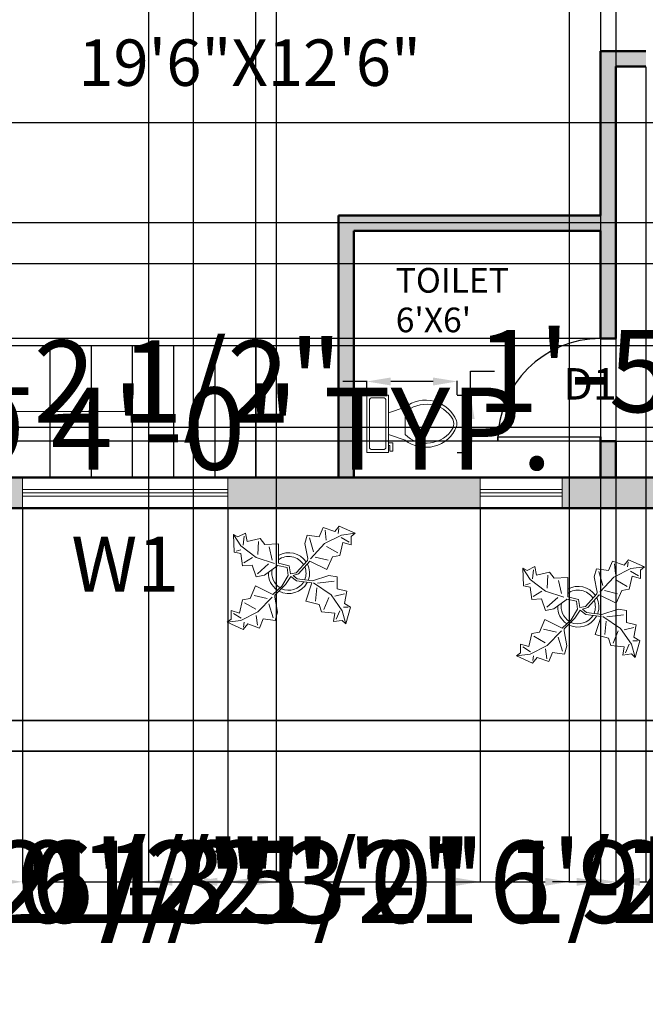
# Model space of a CAD drawing. Units: inches. Extents: x -166 to 1001, y 0 to 688.
# Tile 3 of 11: x 224 to 406, y 0 to 287. Entities that reach past the tile are written whole.
import ezdxf

# ---------------------------------------------------------------- set-up
doc = ezdxf.new("R2010")
doc.units = ezdxf.units.IN
doc.header["$MEASUREMENT"] = 0
for name, color, linetype, lineweight in [('A-ANNO-DIMS', 1, 'Continuous', 18), ('A-ANNO-SYMB', 7, 'Continuous', 18), ('A-ANNO-TEXT', 2, 'Continuous', 25), ('A-AREA-IDEN', 2, 'Continuous', 25), ('A-DOOR', 6, 'Continuous', 25), ('A-FLOR-FIXT', 11, 'Continuous', 18), ('A-FLOR-STRS', 7, 'Continuous', 25), ('A-GLAZ', 130, 'Continuous', 18), ('A-GLAZ-VENT', 130, 'Continuous', 18), ('A-WALL-PATT', 5, 'Continuous', 13), ('C-SITE-WALL', 250, 'Continuous', 35), ('TREES', 80, 'Continuous', 13), ('WALLS', 250, 'Continuous', 50)]:
    doc.layers.add(name, color=color, linetype=linetype, lineweight=lineweight)
doc.styles.get("Standard").update_dxf_attribs({"font": 'arial.ttf'})
doc.dimstyles.get("Standard").update_dxf_attribs({"dimtxt": 24, "dimasz": 7, "dimexe": 0.18, "dimexo": 0.0625, "dimgap": 0.09, "dimtad": 0, "dimtih": 1, "dimtoh": 1, "dimdec": 0, "dimzin": 0, "dimdsep": 46, "dimlunit": 3, "dimtxsty": 'Standard', "dimcen": 0.09, "dimadec": 0, "dimazin": 0, "dimtfac": 1, "dimtdec": 0, "dimtofl": 0, "dimtmove": 0, "dimatfit": 3, "dimfxl": 1, "dimtolj": 1, "dimtzin": 0, "dimarcsym": 0})

# ---------------------------------------------------------------- blocks, each defined once
blk = doc.blocks.new('*U6')
for p, q in [((0, 0), (0, -6)), ((40, 0), (40, -6))]:
    blk.add_line(p, q)
blk.add_lwpolyline([(0, 0), (0, 40), (1.75, 40), (1.75, 0)], close=True)
blk.add_arc((0, 0), 40, 0, 90)
blk = doc.blocks.new('Toilet - top')
for p, q in [((9.5, -6), (9.5, -2)), ((-10, -8.5), (-8, -8.5)), ((-10, -9.5), (-10, -8.5)), ((-7, -9.5), (-10, -9.5)), ((-8, -8.5), (-8, -8)), ((-7, -8), (-7, -9.5)), ((-4, -8), (-6, -14)), ((4, -8), (6, -14)), ((4, -14), (-4, -14))]:
    blk.add_line(p, q)
blk.add_lwpolyline([(10.5, -8), (10.5, 0), (-10.5, 0), (-10.5, -8)], close=True)
for points in [[(-9.5, -2), (-9.5, -6)], [(8.5, -1), (-8.5, -1)], [(-8.5, -7), (8.5, -7)]]:
    blk.add_lwpolyline(points)
for centre, radius, start, end in [((-8.62, -1.88), 0.884, 81.8699, 188.1301), ((8.62, -1.88), 0.884, 351.8699, 98.1301), ((-8.62, -6.12), 0.884, 171.8699, 278.1301), ((8.62, -6.12), 0.884, 261.8699, 8.1301), ((3.52, -21.58), 12.17, 141.4691, 247.9714), ((4.2, -21.82), 11.33, 136.3677, 238.9468), ((-3.52, -21.58), 12.17, 292.0284, 38.5307), ((-4.2, -21.82), 11.33, 301.053, 43.6321), ((0, -27.88), 4, 245.7318, 294.2682), ((0, -29), 4, 254.8605, 285.1395)]:
    blk.add_arc(centre, radius, start, end)
blk = doc.blocks.new('Plant - Rubber or Philodendron')
for p, q in [((-14.8639, 10.7964), (-12.6195, 11.8975)), ((-12.6195, 11.8975), (-12.1909, 9.4345)), ((8.8871, 10.7908), (9.9809, 13.4933)), ((9.9809, 13.4933), (13.3837, 12.301)), ((10.5828, 12.6946), (10.8893, 9.7953)), ((13.3837, 12.301), (14.68, 13.9039)), ((14.5816, 13.2037), (14.3848, 11.8033)), ((14.68, 13.9039), (19.3848, 11.8146)), ((19.3848, 11.8146), (15.3859, 11.3055)), ((19.3848, 11.8146), (18.1868, 10.9119)), ((-16.2005, 11.4774), (-13.9899, 8.1064)), ((-16.2005, 11.4774), (-14.8639, 10.7964)), ((-16.0159, 6.3329), (-16.2005, 11.4774)), ((-13.3174, 8.325), (-13.0735, 11.0065)), ((-12.1909, 9.4345), (-8.3829, 10.3)), ((-8.8369, 9.409), (-9.0894, 5.6095)), ((-8.3829, 10.3), (-7.0549, 8.501)), ((-7.0549, 8.501), (-3.0284, 8.6941)), ((-3.0284, 8.6941), (-3.0709, 3.1041)), ((4.6914, 8.8812), (5.3859, 11.2828)), ((4.6914, 8.8812), (5.5014, 4.4831)), ((5.3859, 11.2828), (8.8871, 10.7908)), ((5.9878, 10.4842), (7.1971, 6.3869)), ((10.3916, 8.7942), (6.2847, 4.4028)), ((15.3859, 11.3055), (10.3916, 8.7942)), ((15.7909, 9.1065), (14.8995, 5.3044)), ((15.2875, 10.6053), (17.5907, 9.2105)), ((18.1925, 8.4119), (15.7909, 9.1065)), ((18.1868, 10.9119), (18.1925, 8.4119)), ((-14.0069, 5.8704), (-16.0159, 6.3329)), ((-15.3434, 6.5514), (-13.9984, 6.9884)), ((-13.5868, 2.2894), (-14.0069, 5.8704)), ((-13.9899, 8.1064), (-9.5434, 4.7185)), ((-4.8529, 4.012), (-5.7184, 7.82)), ((14.2977, 6.1031), (10.9934, 7.9956)), ((-13.1329, 3.1804), (-10.6614, 4.727)), ((-9.5434, 4.7185), (-4.1917, 2.9888)), ((-9.1318, 0.0195), (-5.9793, 2.9025)), ((-3.0709, 3.1041), (0.0797, 2.3163)), ((2.1141, 0.2298), (5.4346, 3.9146)), ((6.1032, 3.6844), (2.8262, -0.031)), ((5.4346, 3.9146), (5.5014, 4.4831)), ((11.1089, 1.1958), (6.1032, 3.6844)), ((7.7005, 4.8881), (11.5025, 3.9967)), ((12.7005, 4.8994), (11.1089, 1.1958)), ((14.8995, 5.3044), (12.7005, 4.8994)), ((-10.6784, 2.491), (-13.5868, 2.2894)), ((-9.5858, -0.8715), (-10.6784, 2.491)), ((-7.1228, -0.443), (-3.5248, 2.2131)), ((-3.5248, 2.2131), (-3.3011, 2.4355)), ((-3.3011, 2.4355), (-0.5306, 1.7947)), ((-0.5306, 1.7947), (-0.2255, -0.5527)), ((-0.5306, 1.7947), (-0.5306, 1.7947)), ((0.0797, 2.3163), (0.4866, -0.031)), ((0.4866, -0.031), (2.1141, 0.2298)), ((-7.1228, -0.443), (-9.5858, -0.8715)), ((-2.019, -3.6148), (-0.2255, -0.5527)), ((-0.9375, -3.1608), (0.5883, -0.8135)), ((0.5883, -0.8135), (2.2447, -2.0916)), ((2.8262, -0.031), (1.3003, -0.5527)), ((1.3003, -0.5527), (2.4193, -1.4655)), ((2.2447, -2.0916), (6.7108, -2.6626)), ((2.4193, -1.4655), (6.895, -2.1175)), ((4.943, -7.9659), (6.7108, -2.6626)), ((11.6605, -0.5413), (6.895, -2.1175)), ((12.3677, -6.1981), (7.219, -2.6772)), ((8.3544, -2.7453), (13.1973, -2.1704)), ((11.6605, -0.5413), (14.1354, -0.8948)), ((14.1354, -0.8948), (14.1354, -4.4304)), ((-11.3237, -7.2629), (-9.7321, -3.5593)), ((-9.7321, -3.5593), (-4.7264, -6.0479)), ((-2.019, -3.6148), (-4.7264, -6.0479)), ((-4.0579, -6.2781), (-0.9375, -3.1608)), ((8.125, -4.0768), (7.7715, -7.9659)), ((14.1354, -4.4304), (16.9638, -5.1375)), ((16.9638, -5.1375), (16.2567, -8.673)), ((-14.4141, -11.4699), (-13.5228, -7.6679)), ((-13.5228, -7.6679), (-11.3237, -7.2629)), ((-12.921, -8.4665), (-9.6166, -10.359)), ((-6.3237, -7.2516), (-10.1257, -6.3602)), ((-9.0148, -11.1577), (-4.9047, -6.8122)), ((-4.1246, -6.8466), (-4.0579, -6.2781)), ((-3.3146, -11.2447), (-4.1246, -6.8466)), ((8.8321, -9.0266), (4.943, -7.9659)), ((10.2463, -10.4408), (11.6605, -6.9053)), ((15.5496, -10.7943), (12.3677, -6.1981)), ((16.2567, -5.8446), (13.4283, -6.5517)), ((-16.8157, -10.7754), (-14.4141, -11.4699)), ((-16.8101, -13.2754), (-16.8157, -10.7754)), ((-14.0091, -13.669), (-9.0148, -11.1577)), ((-4.611, -12.8477), (-5.8203, -8.7504)), ((-3.3146, -11.2447), (-4.0092, -13.6463)), ((9.5392, -11.1479), (8.8321, -9.0266)), ((13.4283, -11.5015), (9.5392, -11.1479)), ((13.0748, -13.9763), (13.4283, -11.5015)), ((14.8425, -10.7943), (13.7819, -13.2692)), ((16.6103, -14.6834), (15.5496, -10.7943)), ((17.3174, -9.7337), (15.9032, -9.7337)), ((16.2567, -8.673), (18.0245, -9.7337)), ((18.0245, -9.7337), (16.6103, -14.6834)), ((-18.008, -14.1781), (-16.8101, -13.2754)), ((-18.008, -14.1781), (-14.0091, -13.669)), ((-13.3032, -16.2674), (-18.008, -14.1781)), ((-13.9107, -12.9688), (-16.2139, -11.574)), ((-13.2048, -15.5672), (-13.008, -14.1668)), ((-9.206, -15.0581), (-9.5126, -12.1588)), ((-7.5103, -13.1543), (-8.6042, -15.8568)), ((-4.0092, -13.6463), (-7.5103, -13.1543)), ((15.5496, -13.6228), (13.0748, -13.9763)), ((16.6103, -14.6834), (15.5496, -13.6228)), ((-12.0069, -14.6645), (-13.3032, -16.2674)), ((-8.6042, -15.8568), (-12.0069, -14.6645))]:
    blk.add_line(p, q)
for centre, radius, start, end in [((0, 0), 6.1275, 34.37569, 120.1028), ((-0.0601, -0.2075), 5.2461, 33.82192, 124.9414), ((0.0308, 0.1664), 6, 178.6147, 235.1169), ((0.0308, 0.1664), 5, 168.1647, 238.6725), ((-0.2664, 0.1682), 5.2775, 338.4094, 20.03007), ((-0.098, 0.1364), 6.1288, 341.2017, 26.09184), ((-0.0234, 0.3825), 6.1492, 242.5812, 331.2714), ((-0.1102, 0.4886), 5.2883, 247.3711, 327.472)]:
    blk.add_arc(centre, radius, start, end)
blk = doc.blocks.new('VENT-24IN')
for p, q in [((0, 4.5), (0, 9)), ((0, 9), (0, 0)), ((24, 9), (24, 0)), ((0, 5.5), (24, 5.5)), ((0, 4.5), (24, 4.5)), ((0, 3.5), (24, 3.5))]:
    blk.add_line(p, q)
blk = doc.blocks.new('*D23')
at = {"layer": 'A-ANNO-DIMS', "color": 0, "lineweight": -2, "transparency": 16777216}
for p, q in [((103.92, 175.12), (103.92, 167.8)), ((151.92, 175.12), (151.92, 167.8)), ((110.92, 167.98), (144.92, 167.98)), ((151.92, 167.98), (158.92, 167.98))]:
    blk.add_line(p, q, dxfattribs=at)
at = {"layer": 'A-ANNO-DIMS', "color": 0, "transparency": 16777216}
for points in [[(110.92, 169.15), (110.92, 166.82), (103.92, 167.98)], [(144.92, 169.15), (144.92, 166.82), (151.92, 167.98)]]:
    blk.add_solid(points, dxfattribs=at)
at = {"layer": 'Defpoints', "color": 0, "transparency": 16777216}
for p in [(103.92, 175.18), (151.92, 175.18), (151.92, 167.98)]:
    blk.add_point(p, dxfattribs=at)
at = {"layer": 'A-ANNO-DIMS', "color": 0, "transparency": 16777216, "insert": (270.75, 167.98), "char_height": 24, "attachment_point": 5}
blk.add_mtext('\\A1;BED 4\'-0" TYP.', dxfattribs=at)
blk = doc.blocks.new('*D27')
at = {"layer": 'A-ANNO-DIMS', "color": 0, "lineweight": -2, "transparency": 16777216}
for p, q in [((325.13, 181.76), (318.13, 181.76)), ((325.13, 177.86), (325.13, 181.94)), ((344.51, 181.76), (332.13, 181.76)), ((351.51, 177.86), (351.51, 181.94))]:
    blk.add_line(p, q, dxfattribs=at)
at = {"layer": 'A-ANNO-DIMS', "color": 0, "transparency": 16777216}
for points in [[(332.13, 182.92), (332.13, 180.59), (325.13, 181.76)], [(344.51, 182.92), (344.51, 180.59), (351.51, 181.76)]]:
    blk.add_solid(points, dxfattribs=at)
at = {"layer": 'Defpoints', "color": 0, "transparency": 16777216}
for p in [(325.13, 181.76), (325.13, 177.8), (351.51, 177.8)]:
    blk.add_point(p, dxfattribs=at)
at = {"layer": 'A-ANNO-DIMS', "color": 0, "transparency": 16777216, "insert": (225.11, 181.76), "char_height": 24, "attachment_point": 5}
blk.add_mtext('\\A1;WC 2\'-2 1/2"', dxfattribs=at)
blk = doc.blocks.new('*D28')
at = {"layer": 'A-ANNO-DIMS', "color": 0, "lineweight": -2, "transparency": 16777216}
for p, q in [((355.46, 177.8), (355.46, 184.8)), ((355.46, 184.8), (362.46, 184.8)), ((351.57, 177.8), (355.64, 177.8)), ((355.46, 168.04), (355.46, 170.8)), ((351.57, 161.04), (355.64, 161.04))]:
    blk.add_line(p, q, dxfattribs=at)
at = {"layer": 'A-ANNO-DIMS', "color": 0, "transparency": 16777216}
for points in [[(354.29, 170.8), (356.63, 170.8), (355.46, 177.8)], [(354.29, 168.04), (356.63, 168.04), (355.46, 161.04)]]:
    blk.add_solid(points, dxfattribs=at)
at = {"layer": 'Defpoints', "color": 0, "transparency": 16777216}
for p in [(351.51, 177.8), (355.46, 177.8), (351.51, 161.04)]:
    blk.add_point(p, dxfattribs=at)
at = {"layer": 'A-ANNO-DIMS', "color": 0, "transparency": 16777216, "insert": (393.32, 184.8), "char_height": 24, "attachment_point": 5}
blk.add_mtext('\\A1;1\'-5"', dxfattribs=at)
blk = doc.blocks.new('*D42')
at = {"layer": 'A-ANNO-DIMS', "color": 0, "lineweight": -2, "transparency": 16777216}
for p, q in [((224.58, 144.68), (224.58, 35.41)), ((284.58, 144.68), (284.58, 35.41)), ((231.58, 35.59), (277.58, 35.59)), ((284.58, 35.59), (291.58, 35.59))]:
    blk.add_line(p, q, dxfattribs=at)
at = {"layer": 'A-ANNO-DIMS', "color": 0, "transparency": 16777216}
for points in [[(231.58, 36.76), (231.58, 34.42), (224.58, 35.59)], [(277.58, 36.76), (277.58, 34.42), (284.58, 35.59)]]:
    blk.add_solid(points, dxfattribs=at)
at = {"layer": 'Defpoints', "color": 0, "transparency": 16777216}
for p in [(224.58, 144.74), (284.58, 144.74), (284.58, 35.59)]:
    blk.add_point(p, dxfattribs=at)
at = {"layer": 'A-ANNO-DIMS', "color": 0, "transparency": 16777216, "insert": (323.57, 35.59), "char_height": 24, "attachment_point": 5}
blk.add_mtext('\\A1;5\'-0"', dxfattribs=at)
blk = doc.blocks.new('*D43')
at = {"layer": 'A-ANNO-DIMS', "color": 0, "lineweight": -2, "transparency": 16777216}
for p, q in [((160.88, 257.49), (160.88, 593.07)), ((167.88, 592.89), (201.62, 592.89)), ((208.62, 257.49), (208.62, 593.07)), ((208.62, 592.89), (215.62, 592.89))]:
    blk.add_line(p, q, dxfattribs=at)
at = {"layer": 'A-ANNO-DIMS', "color": 0, "transparency": 16777216}
for points in [[(167.88, 594.06), (167.88, 591.72), (160.88, 592.89)], [(201.62, 594.06), (201.62, 591.72), (208.62, 592.89)]]:
    blk.add_solid(points, dxfattribs=at)
at = {"layer": 'Defpoints', "color": 0, "transparency": 16777216}
for p in [(208.62, 592.89), (160.88, 257.42), (208.62, 257.42)]:
    blk.add_point(p, dxfattribs=at)
at = {"layer": 'A-ANNO-DIMS', "color": 0, "transparency": 16777216, "insert": (284.89, 592.89), "char_height": 24, "attachment_point": 5}
blk.add_mtext('\\A1;3\'-11 1/2"', dxfattribs=at)
blk = doc.blocks.new('*D44')
at = {"layer": 'A-ANNO-DIMS', "color": 0, "lineweight": -2, "transparency": 16777216}
for p, q in [((144.05, 474.68), (144.05, 35.41)), ((156.38, 474.68), (156.38, 35.41)), ((137.05, 35.59), (130.05, 35.59)), ((163.38, 35.59), (170.38, 35.59))]:
    blk.add_line(p, q, dxfattribs=at)
at = {"layer": 'A-ANNO-DIMS', "color": 0, "transparency": 16777216}
for points in [[(137.05, 36.76), (137.05, 34.42), (144.05, 35.59)], [(163.38, 36.76), (163.38, 34.42), (156.38, 35.59)]]:
    blk.add_solid(points, dxfattribs=at)
at = {"layer": 'Defpoints', "color": 0, "transparency": 16777216}
for p in [(144.05, 474.74), (156.38, 474.74), (156.38, 35.59)]:
    blk.add_point(p, dxfattribs=at)
at = {"layer": 'A-ANNO-DIMS', "color": 0, "transparency": 16777216, "insert": (229.2, 35.59), "char_height": 24, "attachment_point": 5}
blk.add_mtext('\\A1;1\'-0 1/2"', dxfattribs=at)
blk = doc.blocks.new('*D45')
at = {"layer": 'A-ANNO-DIMS', "color": 0, "lineweight": -2, "transparency": 16777216}
for p, q in [((160.88, 474.68), (160.88, 35.41)), ((175.47, 474.68), (175.47, 35.41)), ((167.88, 35.59), (168.47, 35.59)), ((175.47, 35.59), (182.47, 35.59))]:
    blk.add_line(p, q, dxfattribs=at)
at = {"layer": 'A-ANNO-DIMS', "color": 0, "transparency": 16777216}
for points in [[(167.88, 36.76), (167.88, 34.42), (160.88, 35.59)], [(168.47, 36.76), (168.47, 34.42), (175.47, 35.59)]]:
    blk.add_solid(points, dxfattribs=at)
at = {"layer": 'Defpoints', "color": 0, "transparency": 16777216}
for p in [(160.88, 474.74), (175.47, 474.74), (175.47, 35.59)]:
    blk.add_point(p, dxfattribs=at)
at = {"layer": 'A-ANNO-DIMS', "color": 0, "transparency": 16777216, "insert": (241.29, 35.59), "char_height": 24, "attachment_point": 5}
blk.add_mtext('\\A1;1\'-2 1/2"', dxfattribs=at)
blk = doc.blocks.new('*D46')
at = {"layer": 'A-ANNO-DIMS', "color": 0, "lineweight": -2, "transparency": 16777216}
for p, q in [((261.38, 474.68), (261.38, 35.41)), ((298.66, 474.68), (298.66, 35.41)), ((268.38, 35.59), (291.66, 35.59)), ((298.66, 35.59), (305.66, 35.59))]:
    blk.add_line(p, q, dxfattribs=at)
at = {"layer": 'A-ANNO-DIMS', "color": 0, "transparency": 16777216}
for points in [[(268.38, 36.76), (268.38, 34.42), (261.38, 35.59)], [(291.66, 36.76), (291.66, 34.42), (298.66, 35.59)]]:
    blk.add_solid(points, dxfattribs=at)
at = {"layer": 'Defpoints', "color": 0, "transparency": 16777216}
for p in [(261.38, 474.74), (298.66, 474.74), (298.66, 35.59)]:
    blk.add_point(p, dxfattribs=at)
at = {"layer": 'A-ANNO-DIMS', "color": 0, "transparency": 16777216, "insert": (365.61, 35.59), "char_height": 24, "attachment_point": 5}
blk.add_mtext('\\A1;3\'-1 1/2"', dxfattribs=at)
blk = doc.blocks.new('*D49')
at = {"layer": 'A-ANNO-DIMS', "color": 0, "lineweight": -2, "transparency": 16777216}
for p, q in [((149.31, 144.68), (149.31, 35.41)), ((224.58, 144.68), (224.58, 35.41)), ((156.31, 35.59), (217.58, 35.59)), ((224.58, 35.59), (231.58, 35.59))]:
    blk.add_line(p, q, dxfattribs=at)
at = {"layer": 'A-ANNO-DIMS', "color": 0, "transparency": 16777216}
for points in [[(156.31, 36.76), (156.31, 34.42), (149.31, 35.59)], [(217.58, 36.76), (217.58, 34.42), (224.58, 35.59)]]:
    blk.add_solid(points, dxfattribs=at)
at = {"layer": 'Defpoints', "color": 0, "transparency": 16777216}
for p in [(149.31, 144.74), (224.58, 144.74), (224.58, 35.59)]:
    blk.add_point(p, dxfattribs=at)
at = {"layer": 'A-ANNO-DIMS', "color": 0, "transparency": 16777216, "insert": (291.6, 35.59), "char_height": 24, "attachment_point": 5}
blk.add_mtext('\\A1;6\'-3 1/2"', dxfattribs=at)
blk = doc.blocks.new('*D50')
at = {"layer": 'A-ANNO-DIMS', "color": 0, "lineweight": -2, "transparency": 16777216}
for p, q in [((284.58, 144.68), (284.58, 35.41)), ((358.23, 144.68), (358.23, 35.41)), ((291.58, 35.59), (351.23, 35.59)), ((358.23, 35.59), (365.23, 35.59))]:
    blk.add_line(p, q, dxfattribs=at)
at = {"layer": 'A-ANNO-DIMS', "color": 0, "transparency": 16777216}
for points in [[(291.58, 36.76), (291.58, 34.42), (284.58, 35.59)], [(351.23, 36.76), (351.23, 34.42), (358.23, 35.59)]]:
    blk.add_solid(points, dxfattribs=at)
at = {"layer": 'Defpoints', "color": 0, "transparency": 16777216}
for p in [(284.58, 144.74), (358.23, 144.74), (358.23, 35.59)]:
    blk.add_point(p, dxfattribs=at)
at = {"layer": 'A-ANNO-DIMS', "color": 0, "transparency": 16777216, "insert": (425.24, 35.59), "char_height": 24, "attachment_point": 5}
blk.add_mtext('\\A1;6\'-1 1/2"', dxfattribs=at)
blk = doc.blocks.new('*D51')
at = {"layer": 'A-ANNO-DIMS', "color": 0, "lineweight": -2, "transparency": 16777216}
for p, q in [((675.03, 168.41), (675.03, 175.41)), ((675.03, 175.41), (682.03, 175.41)), ((24.44, 168.41), (675.21, 168.41)), ((675.03, 160.74), (675.03, 161.41)), ((24.44, 153.74), (675.21, 153.74))]:
    blk.add_line(p, q, dxfattribs=at)
at = {"layer": 'A-ANNO-DIMS', "color": 0, "transparency": 16777216}
for points in [[(673.87, 161.41), (676.2, 161.41), (675.03, 168.41)], [(673.87, 160.74), (676.2, 160.74), (675.03, 153.74)]]:
    blk.add_solid(points, dxfattribs=at)
at = {"layer": 'Defpoints', "color": 0, "transparency": 16777216}
for p in [(24.38, 168.41), (675.03, 168.41), (24.38, 153.74)]:
    blk.add_point(p, dxfattribs=at)
at = {"layer": 'A-ANNO-DIMS', "color": 0, "transparency": 16777216, "insert": (740.85, 175.41), "char_height": 24, "attachment_point": 5}
blk.add_mtext('\\A1;1\'-2 1/2"', dxfattribs=at)
blk = doc.blocks.new('*D55')
at = {"layer": 'A-ANNO-DIMS', "color": 0, "lineweight": -2, "transparency": 16777216}
for p, q in [((-120.77, 341.73), (-120.77, 348.73)), ((529.82, 334.73), (-120.95, 334.73)), ((529.82, 298.79), (-120.95, 298.79)), ((-120.77, 291.79), (-120.77, 284.79))]:
    blk.add_line(p, q, dxfattribs=at)
at = {"layer": 'A-ANNO-DIMS', "color": 0, "transparency": 16777216}
for points in [[(-121.93, 341.73), (-119.6, 341.73), (-120.77, 334.73)], [(-121.93, 291.79), (-119.6, 291.79), (-120.77, 298.79)]]:
    blk.add_solid(points, dxfattribs=at)
at = {"layer": 'Defpoints', "color": 0, "transparency": 16777216}
for p in [(-120.77, 334.73), (529.88, 334.73), (529.88, 298.79)]:
    blk.add_point(p, dxfattribs=at)
at = {"layer": 'A-ANNO-DIMS', "color": 0, "transparency": 16777216, "insert": (-120.77, 316.76), "char_height": 24, "attachment_point": 5}
blk.add_mtext('\\A1;3\'-0"', dxfattribs=at)
blk = doc.blocks.new('*D60')
at = {"layer": 'A-ANNO-DIMS', "color": 0, "lineweight": -2, "transparency": 16777216}
for p, q in [((156.38, 342.68), (156.38, 35.41)), ((146.03, 338.18), (146.03, 35.41)), ((139.03, 35.59), (132.03, 35.59)), ((163.38, 35.59), (170.38, 35.59))]:
    blk.add_line(p, q, dxfattribs=at)
at = {"layer": 'A-ANNO-DIMS', "color": 0, "transparency": 16777216}
for points in [[(139.03, 36.76), (139.03, 34.42), (146.03, 35.59)], [(163.38, 36.76), (163.38, 34.42), (156.38, 35.59)]]:
    blk.add_solid(points, dxfattribs=at)
at = {"layer": 'Defpoints', "color": 0, "transparency": 16777216}
for p in [(156.38, 342.74), (146.03, 338.24), (156.38, 35.59)]:
    blk.add_point(p, dxfattribs=at)
at = {"layer": 'A-ANNO-DIMS', "color": 0, "transparency": 16777216, "insert": (239.66, 35.59), "char_height": 24, "attachment_point": 5}
blk.add_mtext('\\A1;0\'-10 1/2"', dxfattribs=at)
blk = doc.blocks.new('*D63')
at = {"layer": 'A-ANNO-DIMS', "color": 0, "lineweight": -2, "transparency": 16777216}
for p, q in [((274.49, 338.18), (274.49, 35.41)), ((384.24, 338.18), (384.24, 35.41)), ((281.49, 35.59), (377.24, 35.59)), ((384.24, 35.59), (391.24, 35.59))]:
    blk.add_line(p, q, dxfattribs=at)
at = {"layer": 'A-ANNO-DIMS', "color": 0, "transparency": 16777216}
for points in [[(281.49, 36.76), (281.49, 34.42), (274.49, 35.59)], [(377.24, 36.76), (377.24, 34.42), (384.24, 35.59)]]:
    blk.add_solid(points, dxfattribs=at)
at = {"layer": 'Defpoints', "color": 0, "transparency": 16777216}
for p in [(274.49, 338.24), (384.24, 338.24), (384.24, 35.59)]:
    blk.add_point(p, dxfattribs=at)
at = {"layer": 'A-ANNO-DIMS', "color": 0, "transparency": 16777216, "insert": (451.19, 35.59), "char_height": 24, "attachment_point": 5}
blk.add_mtext('\\A1;9\'-1 1/2"', dxfattribs=at)
blk = doc.blocks.new('*D70')
at = {"layer": 'A-ANNO-DIMS', "color": 0, "lineweight": -2, "transparency": 16777216}
for p, q in [((147.87, 273.68), (147.87, 35.41)), ((156.38, 273.68), (156.38, 35.41)), ((140.87, 35.59), (133.87, 35.59)), ((163.38, 35.59), (170.38, 35.59))]:
    blk.add_line(p, q, dxfattribs=at)
at = {"layer": 'A-ANNO-DIMS', "color": 0, "transparency": 16777216}
for points in [[(140.87, 36.76), (140.87, 34.42), (147.87, 35.59)], [(163.38, 36.76), (163.38, 34.42), (156.38, 35.59)]]:
    blk.add_solid(points, dxfattribs=at)
at = {"layer": 'Defpoints', "color": 0, "transparency": 16777216}
for p in [(147.87, 273.74), (156.38, 273.74), (156.38, 35.59)]:
    blk.add_point(p, dxfattribs=at)
at = {"layer": 'A-ANNO-DIMS', "color": 0, "transparency": 16777216, "insert": (230.33, 35.59), "char_height": 24, "attachment_point": 5}
blk.add_mtext('\\A1;0\'-8 1/2"', dxfattribs=at)
blk = doc.blocks.new('*D72')
at = {"layer": 'A-ANNO-DIMS', "color": 0, "lineweight": -2, "transparency": 16777216}
for p, q in [((397.88, 273.68), (397.88, 35.41)), ((406.66, 273.68), (406.66, 35.41)), ((390.88, 35.59), (383.88, 35.59)), ((413.66, 35.59), (420.66, 35.59))]:
    blk.add_line(p, q, dxfattribs=at)
at = {"layer": 'A-ANNO-DIMS', "color": 0, "transparency": 16777216}
for points in [[(390.88, 36.76), (390.88, 34.42), (397.88, 35.59)], [(413.66, 36.76), (413.66, 34.42), (406.66, 35.59)]]:
    blk.add_solid(points, dxfattribs=at)
at = {"layer": 'Defpoints', "color": 0, "transparency": 16777216}
for p in [(397.88, 273.74), (406.66, 273.74), (406.66, 35.59)]:
    blk.add_point(p, dxfattribs=at)
at = {"layer": 'A-ANNO-DIMS', "color": 0, "transparency": 16777216, "insert": (452.65, 35.59), "char_height": 24, "attachment_point": 5}
blk.add_mtext('\\A1;0\'-9"', dxfattribs=at)
blk = doc.blocks.new('*D73')
at = {"layer": 'A-ANNO-DIMS', "color": 0, "lineweight": -2, "transparency": 16777216}
for p, q in [((-120.77, 201.32), (-120.77, 208.32)), ((393.32, 194.32), (-120.95, 194.32)), ((393.32, 164.32), (-120.95, 164.32)), ((-120.77, 157.32), (-120.77, 150.32))]:
    blk.add_line(p, q, dxfattribs=at)
at = {"layer": 'A-ANNO-DIMS', "color": 0, "transparency": 16777216}
for points in [[(-121.93, 201.32), (-119.6, 201.32), (-120.77, 194.32)], [(-121.93, 157.32), (-119.6, 157.32), (-120.77, 164.32)]]:
    blk.add_solid(points, dxfattribs=at)
at = {"layer": 'Defpoints', "color": 0, "transparency": 16777216}
for p in [(-120.77, 194.32), (393.38, 194.32), (393.38, 164.32)]:
    blk.add_point(p, dxfattribs=at)
at = {"layer": 'A-ANNO-DIMS', "color": 0, "transparency": 16777216, "insert": (-120.77, 179.32), "char_height": 24, "attachment_point": 5}
blk.add_mtext('\\A1;2\'-6"', dxfattribs=at)
blk = doc.blocks.new('*D74')
at = {"layer": 'A-ANNO-DIMS', "color": 0, "lineweight": -2, "transparency": 16777216}
for p, q in [((675.03, 171.32), (675.03, 178.32)), ((675.03, 178.32), (682.03, 178.32)), ((397.94, 164.32), (675.21, 164.32)), ((397.94, 153.74), (675.21, 153.74)), ((675.03, 146.74), (675.03, 139.74))]:
    blk.add_line(p, q, dxfattribs=at)
at = {"layer": 'A-ANNO-DIMS', "color": 0, "transparency": 16777216}
for points in [[(673.87, 171.32), (676.2, 171.32), (675.03, 164.32)], [(673.87, 146.74), (676.2, 146.74), (675.03, 153.74)]]:
    blk.add_solid(points, dxfattribs=at)
at = {"layer": 'Defpoints', "color": 0, "transparency": 16777216}
for p in [(397.88, 164.32), (675.03, 164.32), (397.88, 153.74)]:
    blk.add_point(p, dxfattribs=at)
at = {"layer": 'A-ANNO-DIMS', "color": 0, "transparency": 16777216, "insert": (751.31, 178.32), "char_height": 24, "attachment_point": 5}
blk.add_mtext('\\A1;0\'-10 1/2"', dxfattribs=at)
blk = doc.blocks.new('*D76')
at = {"layer": 'A-ANNO-DIMS', "color": 0, "lineweight": -2, "transparency": 16777216}
for p, q in [((675.03, 235.24), (675.03, 242.24)), ((160.94, 228.24), (675.21, 228.24)), ((160.94, 216.24), (675.21, 216.24)), ((675.03, 209.24), (675.03, 202.24)), ((675.03, 202.24), (668.03, 202.24))]:
    blk.add_line(p, q, dxfattribs=at)
at = {"layer": 'A-ANNO-DIMS', "color": 0, "transparency": 16777216}
for points in [[(673.87, 235.24), (676.2, 235.24), (675.03, 228.24)], [(673.87, 209.24), (676.2, 209.24), (675.03, 216.24)]]:
    blk.add_solid(points, dxfattribs=at)
at = {"layer": 'Defpoints', "color": 0, "transparency": 16777216}
for p in [(160.88, 228.24), (160.88, 216.24), (675.03, 216.24)]:
    blk.add_point(p, dxfattribs=at)
at = {"layer": 'A-ANNO-DIMS', "color": 0, "transparency": 16777216, "insert": (637.17, 202.24), "char_height": 24, "attachment_point": 5}
blk.add_mtext('\\A1;1\'-0"', dxfattribs=at)
blk = doc.blocks.new('*D77')
at = {"layer": 'A-ANNO-DIMS', "color": 0, "lineweight": -2, "transparency": 16777216}
for p, q in [((675.03, 199.24), (675.03, 206.24)), ((292.83, 192.24), (675.21, 192.24)), ((292.83, 153.74), (675.21, 153.74)), ((675.03, 146.74), (675.03, 139.74))]:
    blk.add_line(p, q, dxfattribs=at)
at = {"layer": 'A-ANNO-DIMS', "color": 0, "transparency": 16777216}
for points in [[(673.87, 199.24), (676.2, 199.24), (675.03, 192.24)], [(673.87, 146.74), (676.2, 146.74), (675.03, 153.74)]]:
    blk.add_solid(points, dxfattribs=at)
at = {"layer": 'Defpoints', "color": 0, "transparency": 16777216}
for p in [(292.77, 192.24), (292.77, 153.74), (675.03, 153.74)]:
    blk.add_point(p, dxfattribs=at)
at = {"layer": 'A-ANNO-DIMS', "color": 0, "transparency": 16777216, "insert": (675.03, 172.99), "char_height": 24, "attachment_point": 5}
blk.add_mtext('\\A1;3\'-2 1/2"', dxfattribs=at)
blk = doc.blocks.new('*D78')
at = {"layer": 'A-ANNO-DIMS', "color": 0, "lineweight": -2, "transparency": 16777216}
for p, q in [((160.88, 153.8), (160.88, 593.07)), ((167.88, 592.89), (186.64, 592.89)), ((285.77, 592.89), (267.01, 592.89)), ((292.77, 153.8), (292.77, 593.07))]:
    blk.add_line(p, q, dxfattribs=at)
at = {"layer": 'A-ANNO-DIMS', "color": 0, "transparency": 16777216}
for points in [[(167.88, 594.06), (167.88, 591.72), (160.88, 592.89)], [(285.77, 594.06), (285.77, 591.72), (292.77, 592.89)]]:
    blk.add_solid(points, dxfattribs=at)
at = {"layer": 'Defpoints', "color": 0, "transparency": 16777216}
for p in [(292.77, 592.89), (160.88, 153.74), (292.77, 153.74)]:
    blk.add_point(p, dxfattribs=at)
at = {"layer": 'A-ANNO-DIMS', "color": 0, "transparency": 16777216, "insert": (226.83, 592.89), "char_height": 24, "attachment_point": 5}
blk.add_mtext('\\A1;11\'-0"', dxfattribs=at)
blk = doc.blocks.new('*D79')
at = {"layer": 'A-ANNO-DIMS', "color": 0, "lineweight": -2, "transparency": 16777216}
for p, q in [((208.68, 257.42), (675.21, 257.42)), ((675.03, 250.42), (675.03, 218.08)), ((675.03, 160.74), (675.03, 193.08)), ((292.83, 153.74), (675.21, 153.74))]:
    blk.add_line(p, q, dxfattribs=at)
at = {"layer": 'A-ANNO-DIMS', "color": 0, "transparency": 16777216}
for points in [[(673.87, 250.42), (676.2, 250.42), (675.03, 257.42)], [(673.87, 160.74), (676.2, 160.74), (675.03, 153.74)]]:
    blk.add_solid(points, dxfattribs=at)
at = {"layer": 'Defpoints', "color": 0, "transparency": 16777216}
for p in [(208.62, 257.42), (292.77, 153.74), (675.03, 153.74)]:
    blk.add_point(p, dxfattribs=at)
at = {"layer": 'A-ANNO-DIMS', "color": 0, "transparency": 16777216, "insert": (675.03, 205.58), "char_height": 24, "attachment_point": 5}
blk.add_mtext('\\A1;8\'-7 1/2"', dxfattribs=at)
blk = doc.blocks.new('*D80')
at = {"layer": 'A-ANNO-DIMS', "color": 0, "lineweight": -2, "transparency": 16777216}
for p, q in [((393.38, 383.15), (393.38, 35.41)), ((397.88, 383.15), (397.88, 35.41)), ((386.38, 35.59), (379.38, 35.59)), ((404.88, 35.59), (411.88, 35.59))]:
    blk.add_line(p, q, dxfattribs=at)
at = {"layer": 'A-ANNO-DIMS', "color": 0, "transparency": 16777216}
for points in [[(386.38, 36.76), (386.38, 34.42), (393.38, 35.59)], [(404.88, 36.76), (404.88, 34.42), (397.88, 35.59)]]:
    blk.add_solid(points, dxfattribs=at)
at = {"layer": 'Defpoints', "color": 0, "transparency": 16777216}
for p in [(393.38, 383.21), (397.88, 383.21), (397.88, 35.59)]:
    blk.add_point(p, dxfattribs=at)
at = {"layer": 'A-ANNO-DIMS', "color": 0, "transparency": 16777216, "insert": (471.83, 35.59), "char_height": 24, "attachment_point": 5}
blk.add_mtext('\\A1;0\'-4 1/2"', dxfattribs=at)

msp = doc.modelspace()

# ---------------------------------------------------------------- hatches: boundary and pattern name
at = {"layer": 'A-WALL-PATT'}
h = msp.add_hatch(color=256, dxfattribs=at)
h.dxf.hatch_style = 1
h.paths.add_polyline_path([(96.05, 483.74), (15.38, 483.74), (15.38, 414.29), (24.38, 414.29), (24.38, 474.74), (96.05, 474.74)])
h.paths.add_polyline_path([(175.47, 483.74), (144.05, 483.74), (144.05, 474.74), (156.38, 474.74), (175.47, 474.74)])
h.paths.add_polyline_path([(298.66, 483.74), (199.47, 483.74), (199.47, 474.74), (256.88, 474.74), (298.66, 474.74)])
h.paths.add_polyline_path([(430.46, 483.74), (346.66, 483.74), (346.66, 474.74), (393.38, 474.74), (430.46, 474.74)])
h.paths.add_polyline_path([(261.38, 474.74), (256.88, 474.74), (256.88, 342.74), (201.55, 342.74), (201.55, 338.24), (274.49, 338.24), (274.49, 342.74), (261.38, 342.74)])
h.paths.add_polyline_path([(160.88, 474.74), (156.38, 474.74), (156.38, 342.74), (146.03, 342.74), (146.03, 338.24), (171.55, 338.24), (171.55, 342.74), (160.88, 342.74)])
h.paths.add_polyline_path([(397.88, 474.74), (393.38, 474.74), (393.38, 383.21), (397.88, 383.21)])
h.paths.add_polyline_path([(538.88, 362.18), (529.88, 362.18), (529.88, 342.74), (397.88, 342.74), (397.88, 348.69), (393.38, 348.69), (393.38, 342.74), (384.24, 342.74), (384.24, 338.24), (529.88, 338.24), (529.88, 334.73), (538.88, 334.73)])
h.paths.add_polyline_path([(538.88, 483.74), (478.46, 483.74), (478.46, 474.74), (529.88, 474.74), (529.88, 410.18), (538.88, 410.18)])
h.paths.add_polyline_path([(538.88, 298.79), (529.88, 298.79), (529.88, 278.24), (442.61, 278.24), (442.61, 273.74), (529.88, 273.74), (529.88, 221.94), (538.88, 221.94)])
h.paths.add_polyline_path([(538.88, 173.94), (529.88, 173.94), (529.88, 153.74), (393.38, 153.74), (382.23, 153.74), (382.23, 144.74), (538.88, 144.74)])
h.paths.add_polyline_path([(397.88, 164.32), (393.38, 164.32), (393.38, 153.74), (397.88, 153.74)], flags=17)
h.paths.add_polyline_path([(397.88, 273.74), (406.66, 273.74), (406.66, 278.24), (393.38, 278.24), (393.38, 273.74), (393.38, 230.24), (316.88, 230.24), (316.88, 153.74), (321.38, 153.74), (321.38, 225.74), (393.38, 225.74), (393.38, 194.32), (397.88, 194.32)])
h.paths.add_polyline_path([(358.23, 153.74), (316.88, 153.74), (284.58, 153.74), (284.58, 144.74), (358.23, 144.74)])
h.paths.add_polyline_path([(224.58, 153.74), (156.38, 153.74), (149.31, 153.74), (149.31, 144.74), (224.58, 144.74)])
h.paths.add_polyline_path([(101.31, 153.74), (24.38, 153.74), (24.38, 168.41), (15.38, 168.41), (15.38, 144.74), (101.31, 144.74)])
h.paths.add_polyline_path([(160.88, 273.74), (160.88, 278.24), (147.87, 278.24), (147.87, 273.74), (156.38, 273.74), (156.38, 153.74), (160.88, 153.74)])
h.paths.add_polyline_path([(111.92, 278.24), (100.88, 278.24), (100.88, 338.24), (110.03, 338.24), (110.03, 342.74), (24.38, 342.74), (24.38, 366.29), (15.38, 366.29), (15.38, 216.41), (24.38, 216.41), (24.38, 273.74), (44.93, 273.74), (44.93, 278.24), (24.38, 278.24), (24.38, 338.24), (96.38, 338.24), (96.38, 278.24), (74.93, 278.24), (74.93, 273.74), (111.92, 273.74)])

# ---------------------------------------------------------------- linework, layer by layer
at = {"layer": 'A-ANNO-SYMB'}
msp.add_line((256.68, 172.99), (184.73, 172.99), dxfattribs=at)
at = {"layer": 'A-FLOR-STRS'}
for p, q in [((208.62, 192.24), (292.77, 192.24)), ((232.63, 192.24), (232.63, 153.74)), ((244.66, 192.24), (244.66, 153.74)), ((256.68, 192.24), (256.68, 153.74)), ((268.71, 192.24), (268.71, 153.74)), ((280.74, 192.24), (280.74, 153.74)), ((292.77, 192.24), (292.77, 153.74))]:
    msp.add_line(p, q, dxfattribs=at)
at = {"layer": 'A-GLAZ'}
for p, q in [((224.58, 149.24), (224.58, 153.74)), ((224.58, 153.74), (224.58, 144.74)), ((284.58, 153.74), (284.58, 144.74)), ((224.58, 150.24), (284.58, 150.24)), ((224.58, 149.24), (284.58, 149.24)), ((224.58, 148.24), (284.58, 148.24))]:
    msp.add_line(p, q, dxfattribs=at)
at = {"layer": 'C-SITE-WALL'}
for p, q in [((-73.62, 82.74), (627.88, 82.74)), ((-82.62, 73.74), (636.88, 73.74))]:
    msp.add_line(p, q, dxfattribs=at)
at = {"layer": 'WALLS'}
for p, q in [((393.38, 278.24), (406.66, 278.24)), ((393.38, 273.74), (393.38, 278.24)), ((393.38, 230.24), (393.38, 273.74)), ((397.88, 273.74), (406.66, 273.74)), ((397.88, 194.32), (397.88, 273.74)), ((316.88, 153.74), (316.88, 230.24)), ((316.88, 230.24), (393.38, 230.24)), ((321.38, 153.74), (321.38, 225.74)), ((321.38, 225.74), (393.38, 225.74)), ((393.38, 194.32), (393.38, 225.74)), ((393.38, 194.32), (397.88, 194.32)), ((393.38, 153.74), (393.38, 165.63)), ((393.38, 164.32), (397.88, 164.32)), ((397.88, 153.74), (397.88, 164.32)), ((156.38, 153.74), (316.88, 153.74)), ((316.88, 153.74), (393.38, 153.74)), ((393.38, 153.74), (529.88, 153.74)), ((15.38, 144.74), (538.88, 144.74))]:
    msp.add_line(p, q, dxfattribs=at)

# ---------------------------------------------------------------- block references
at = {"layer": 'A-DOOR', "xscale": 0.7500000000000006, "yscale": 0.7500000000000006, "zscale": 0.7500000000000006, "rotation": 90}
msp.add_blockref('*U6', (393.38, 164.32), dxfattribs=at)
at = {"layer": 'A-FLOR-FIXT', "xscale": 0.7980112901843065, "yscale": 0.7980112901843065, "zscale": 0.7980112901843065, "rotation": 90}
msp.add_blockref('Toilet - top', (325.13, 169.42), dxfattribs=at)
at = {"layer": 'A-GLAZ-VENT'}
msp.add_blockref('VENT-24IN', (358.23, 144.74), dxfattribs=at)
at = {"layer": 'TREES'}
for p in [(302.39, 125.59), (386.87, 115.77)]:
    msp.add_blockref('Plant - Rubber or Philodendron', p, dxfattribs=at)

# ---------------------------------------------------------------- texts
at = {"layer": 'A-ANNO-TEXT'}
for s, height, p in [('D1', 9.17, (382.55, 176.48)), ('W1 ', 16.096, (238.86, 120.34))]:
    msp.add_text(s, height=height, dxfattribs=at).set_placement(p)
at = {"layer": 'A-AREA-IDEN'}
for s, height, p in [('19\'6"X12\'6"', 13.5669, (240.9, 268.11)), ('TOILET', 7.198, (333.6, 207.71)), ("6'X6'", 7.198, (333.6, 196.14))]:
    msp.add_text(s, height=height, dxfattribs=at).set_placement(p)

# ---------------------------------------------------------------- dimensions: what is measured, and where the dimension line sits
at = {"layer": 'A-ANNO-DIMS'}
for base, p1, p2, picture, middle in [((208.62, 592.89), (160.88, 257.42), (208.62, 257.42), '*D43', (284.89, 592.89)), ((292.77, 592.89), (160.88, 153.74), (292.77, 153.74), '*D78', (226.83, 592.89)), ((156.38, 35.59), (144.05, 474.74), (156.38, 474.74), '*D44', (229.2, 35.59)), ((175.47, 35.59), (160.88, 474.74), (175.47, 474.74), '*D45', (241.29, 35.59)), ((298.66, 35.59), (261.38, 474.74), (298.66, 474.74), '*D46', (365.61, 35.59)), ((397.88, 35.59), (393.38, 383.21), (397.88, 383.21), '*D80', (471.83, 35.59)), ((156.3825, 35.5909), (146.0262, 338.2409), (156.3825, 342.7409), '*D60', (239.6566, 35.5909)), ((384.2404, 35.5909), (274.4932, 338.2409), (384.2404, 338.2409), '*D63', (451.1912, 35.5909)), ((156.38, 35.59), (147.87, 273.74), (156.38, 273.74), '*D70', (230.33, 35.59)), ((406.66, 35.59), (397.88, 273.74), (406.66, 273.74), '*D72', (452.65, 35.59)), ((224.58, 35.59), (149.31, 144.74), (224.58, 144.74), '*D49', (291.6, 35.59)), ((284.58, 35.59), (224.58, 144.74), (284.58, 144.74), '*D42', (323.57, 35.59)), ((358.2261, 35.5909), (284.5839, 144.7409), (358.2261, 144.7409), '*D50', (425.2425, 35.5909))]:
    dim = msp.add_linear_dim(base=base, p1=p1, p2=p2, dimstyle='Standard', override={"dimdec": 1, "dimlfac": 1, "dimrnd": 0, "dimzin": 1, "dimdsep": 46, "dimlunit": 4, "dimfrac": 2}, dxfattribs=at)
    dim.commit()
    dim.dimension.update_dxf_attribs({"geometry": picture, "text_midpoint": middle})
for base, p1, p2, picture, middle in [((-120.77, 334.73), (529.88, 298.79), (529.88, 334.73), '*D55', (-120.77, 316.76)), ((675.03, 153.74), (208.62, 257.42), (292.77, 153.74), '*D79', (675.03, 205.58)), ((675.03, 216.24), (160.88, 228.24), (160.88, 216.24), '*D76', (637.17, 202.24)), ((675.03, 164.32), (397.88, 153.74), (397.88, 164.32), '*D74', (751.31, 178.32)), ((675.03, 168.41), (24.38, 153.74), (24.38, 168.41), '*D51', (740.85, 175.41)), ((-120.77, 194.32), (393.38, 164.32), (393.38, 194.32), '*D73', (-120.77, 179.32)), ((675.03, 153.74), (292.77, 192.24), (292.77, 153.74), '*D77', (675.03, 172.99)), ((355.46, 177.8), (351.51, 161.04), (351.51, 177.8), '*D28', (393.32, 184.8))]:
    dim = msp.add_linear_dim(base=base, p1=p1, p2=p2, angle=90, dimstyle='Standard', override={"dimdec": 1, "dimlfac": 1, "dimrnd": 0, "dimzin": 1, "dimdsep": 46, "dimlunit": 4, "dimfrac": 2}, dxfattribs=at)
    dim.commit()
    dim.dimension.update_dxf_attribs({"geometry": picture, "text_midpoint": middle})
dim = msp.add_linear_dim(base=(325.13, 181.76), p1=(351.51, 177.8), p2=(325.13, 177.8), angle=180, text='WC <>', dimstyle='Standard', override={"dimdec": 1, "dimlfac": 1, "dimrnd": 0, "dimzin": 1, "dimdsep": 46, "dimlunit": 4, "dimfrac": 2}, dxfattribs=at)
dim.commit()
dim.dimension.update_dxf_attribs({"geometry": '*D27', "text_midpoint": (225.11, 181.76)})
dim = msp.add_linear_dim(base=(151.92, 167.98), p1=(103.92, 175.18), p2=(151.92, 175.18), text='BED <> TYP.', dimstyle='Standard', override={"dimdec": 1, "dimlfac": 1, "dimrnd": 0, "dimzin": 1, "dimdsep": 46, "dimlunit": 4, "dimfrac": 2}, dxfattribs=at)
dim.commit()
dim.dimension.update_dxf_attribs({"geometry": '*D23', "text_midpoint": (270.75, 167.98)})

doc.saveas('drawing.dxf')
